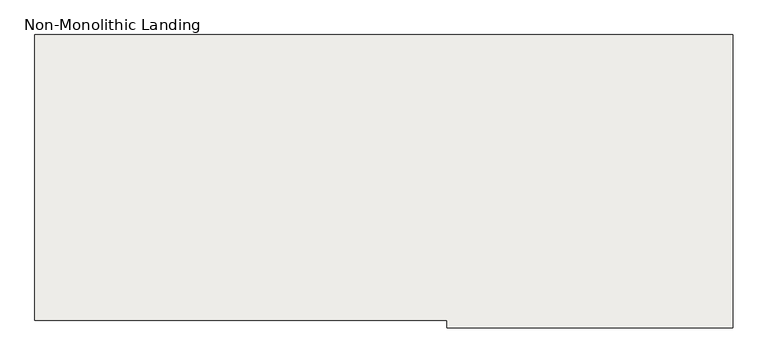
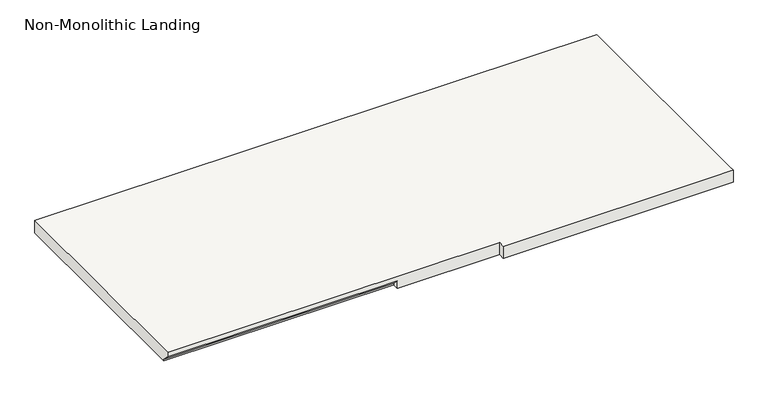
"""IFC4 building model written with IfcOpenShell, lengths in millimetres: slab geometry, Non-Monolithic Landing."""

from ifc_helpers import new_model, si_unit, origin, place, context, project, spatial, faceted_brep, source, transform, mapped, element, save


def non_monolithic_landing_8e40c115(model_context):
    return source(origin(), model_context, "Body", "Brep", [
        faceted_brep([(-3617.4415084, -19522.1851539, 48922.2339133), (-3617.4415084, -19496.7851539, 48896.8339133), (-2703.0415084, -19496.7851539, 48896.8339133), (-2703.0415084, -19522.1851539, 48922.2339133), (-2296.6415084, -19522.1851539, 48941.2839133), (-2296.6415084, -19547.5851539, 48941.2839133), (-1382.2415084, -19547.5851539, 48941.2839133), (-1382.2415084, -19522.1851539, 48941.2839133), (-1382.2415084, -18607.7851539, 48941.2839133), (-3617.4415084, -18607.7851539, 48941.2839133), (-3617.4415084, -19522.1851539, 48941.2839133), (-2703.0415084, -19496.7851539, 48890.4839133), (-3617.4415084, -19496.7851539, 48890.4839133), (-3617.4415084, -18607.7851539, 48890.4839133), (-1382.2415084, -18607.7851539, 48890.4839133), (-1382.2415084, -19522.1851539, 48890.4839133), (-1382.2415084, -19547.5851539, 48890.4839133), (-2296.6415084, -19547.5851539, 48890.4839133), (-2296.6415084, -19522.1851539, 48890.4839133), (-2703.0415084, -19522.1851539, 48890.4839133)], [[[0, 1, 2, 3]], [[4, 5, 6, 7, 8, 9, 10]], [[11, 12, 13, 14, 15, 16, 17, 18, 19]], [[12, 11, 2, 1]], [[11, 19, 3, 2]], [[4, 10, 0, 3, 19, 18]], [[5, 4, 18, 17]], [[6, 5, 17, 16]], [[7, 6, 16, 15]], [[8, 7, 15, 14]], [[9, 8, 14, 13]], [[10, 9, 13, 12, 1, 0]]]),
    ])


if __name__ == "__main__":
    model = new_model("IFC4")
    model_context = context("Model", 3, world=origin())
    ifc_project = project(units=[si_unit("LENGTHUNIT", "METRE", prefix="MILLI")], contexts=[model_context])
    site = spatial("IfcSite", under=ifc_project)
    building = spatial("IfcBuilding", under=site)
    placement = place(None, origin())
    non_monolithic_landing_shape = non_monolithic_landing_8e40c115(model_context)
    element("IfcSlab", 1, ObjectType="Non-Monolithic Landing", at=placement, inside=building, context=model_context, shape_type="MappedRepresentation", body=[
        mapped(non_monolithic_landing_shape, transform((0.0, 0.0, 0.0), x_axis=(1.0, 0.0, 0.0), y_axis=(0.0, 1.0, 0.0), z_axis=(0.0, 0.0, 1.0))),
    ])
    save(model, "model.ifc")
